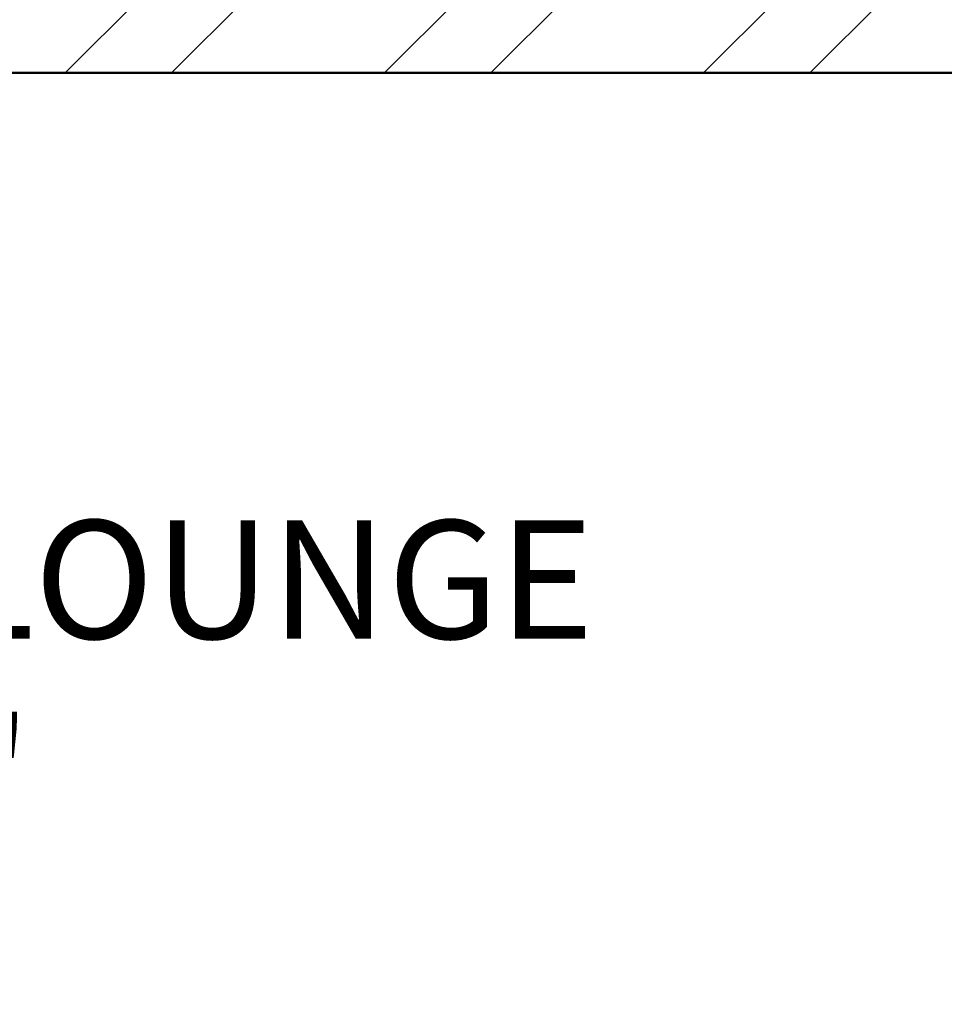
# Model space of a CAD drawing. Units: inches. Extents: x 963 to 2075, y 289 to 2657.
# Tile 91 of 98: x 1728 to 1767, y 2283 to 2325. Entities that reach past the tile are written whole.
import ezdxf

# ---------------------------------------------------------------- set-up
doc = ezdxf.new("R2010")
doc.units = ezdxf.units.IN
for name, color, linetype, lineweight in [('A-AREA-IDEN', 7, 'Continuous', 18), ('A-WALL', 7, 'Continuous', 50), ('A-WALL-PATT', 8, 'Continuous', 13)]:
    doc.layers.add(name, color=color, linetype=linetype, lineweight=lineweight)
doc.styles.get("Standard").update_dxf_attribs({"font": 'arial.ttf'})

msp = doc.modelspace()

# ---------------------------------------------------------------- hatches: boundary and pattern name
at = {"layer": 'A-WALL-PATT'}
h = msp.add_hatch(dxfattribs=at)
h.set_pattern_fill('ANSI32', color=256)
h.paths.add_polyline_path([(1296.922, 2558.318), (1203.922, 2558.318), (1203.922, 2493.818), (1191.533, 2493.818), (1191.533, 2489.318), (1211.063, 2489.318), (1211.063, 2492.02), (1211.063, 2493.818), (1208.422, 2493.818), (1208.422, 2553.818), (1292.422, 2553.818), (1292.422, 2538.863), (1296.922, 2538.863)])
h.paths.add_polyline_path([(1442.422, 2558.318), (1349.422, 2558.318), (1349.422, 2538.943), (1353.922, 2538.943), (1353.922, 2553.818), (1437.922, 2553.818), (1437.922, 2493.818), (1434.542, 2493.818), (1434.542, 2489.318), (1448.311, 2489.318), (1448.311, 2491.568), (1448.311, 2493.818), (1442.422, 2493.818)])
h.paths.add_polyline_path([(1415.554, 2491.568), (1415.554, 2493.818), (1340.941, 2493.818), (1340.941, 2489.318), (1371.922, 2489.318), (1371.922, 2378.318), (1367.596, 2378.318), (1367.596, 2373.818), (1371.922, 2373.818), (1371.922, 2355.185), (1376.422, 2355.185), (1376.422, 2489.318), (1415.554, 2489.318)])
h.paths.add_polyline_path([(1304.941, 2491.568), (1304.941, 2493.818), (1296.922, 2493.818), (1296.922, 2514.863), (1292.422, 2514.863), (1292.422, 2493.818), (1232.808, 2493.818), (1232.808, 2489.318), (1256.422, 2489.318), (1256.422, 2327.318), (1253.714, 2327.318), (1253.714, 2322.818), (1328.422, 2322.818), (1328.422, 2331.147), (1323.922, 2331.147), (1323.922, 2327.318), (1260.922, 2327.318), (1260.922, 2373.818), (1323.922, 2373.818), (1323.922, 2357.812), (1328.422, 2357.812), (1328.422, 2373.818), (1346.007, 2373.818), (1346.007, 2376.068), (1346.007, 2378.318), (1260.922, 2378.318), (1260.922, 2489.318), (1304.941, 2489.318)])
h.paths.add_polyline_path([(1226.654, 2327.318), (1124.422, 2327.318), (1124.422, 2347.447), (1119.922, 2347.447), (1119.922, 2322.818), (1163.422, 2322.818), (1163.422, 2305.435), (1165.672, 2305.435), (1167.922, 2305.435), (1167.922, 2322.818), (1226.654, 2322.818), (1226.654, 2325.068)])
h.paths.add_polyline_path([(1095.922, 2489.318), (1124.422, 2489.318), (1131.533, 2489.318), (1131.533, 2491.568), (1131.533, 2493.818), (1119.922, 2493.818), (1091.422, 2493.818), (1091.422, 2417.318), (1095.922, 2417.318), (1119.922, 2417.318), (1119.922, 2407.447), (1124.422, 2407.447), (1124.422, 2421.818), (1095.922, 2421.818)])
h.paths.add_polyline_path([(1512.922, 2558.318), (1508.422, 2558.318), (1508.422, 2493.818), (1503.401, 2493.818), (1503.401, 2489.318), (1508.422, 2489.318), (1508.422, 2327.318), (1376.422, 2327.318), (1376.422, 2330.273), (1371.922, 2330.273), (1371.922, 2298.744), (1376.422, 2298.744), (1376.422, 2322.818), (1508.422, 2322.818), (1508.422, 2165.318), (1504.255, 2165.318), (1504.255, 2160.818), (1508.422, 2160.818), (1508.422, 2108.318), (1512.922, 2108.318), (1512.922, 2160.818), (1516.182, 2160.818), (1516.182, 2163.068), (1516.182, 2165.318), (1512.922, 2165.318), (1512.922, 2322.818), (1644.922, 2322.818), (1644.922, 2298.744), (1649.422, 2298.744), (1649.422, 2322.818), (1649.422, 2330.944), (1647.172, 2330.944), (1644.922, 2330.944), (1644.922, 2327.318), (1512.922, 2327.318), (1512.922, 2489.318), (1516.759, 2489.318), (1516.759, 2491.568), (1516.759, 2493.818), (1512.922, 2493.818)])
h.paths.add_polyline_path([(1671.922, 2558.318), (1578.922, 2558.318), (1578.922, 2493.818), (1573.526, 2493.818), (1573.526, 2489.318), (1586.537, 2489.318), (1586.537, 2491.568), (1586.537, 2493.818), (1583.422, 2493.818), (1583.422, 2553.818), (1667.422, 2553.818), (1667.422, 2541.109), (1671.922, 2541.109)])
h.paths.add_polyline_path([(1681.257, 2493.818), (1671.922, 2493.818), (1671.922, 2517.109), (1667.422, 2517.109), (1667.422, 2493.818), (1610.218, 2493.818), (1610.218, 2489.318), (1644.922, 2489.318), (1644.922, 2357.865), (1649.422, 2357.865), (1649.422, 2373.818), (1652.203, 2373.818), (1652.203, 2375.827), (1652.203, 2378.318), (1649.422, 2378.318), (1649.422, 2489.318), (1681.257, 2489.318), (1681.257, 2491.568)])
h.paths.add_polyline_path([(1821.922, 2558.318), (1728.922, 2558.318), (1728.922, 2541), (1733.422, 2541), (1733.422, 2553.818), (1817.422, 2553.818), (1817.422, 2493.818), (1813.507, 2493.818), (1813.507, 2489.318), (1830.078, 2489.318), (1830.078, 2491.568), (1830.078, 2493.818), (1821.922, 2493.818)])
h.paths.add_polyline_path([(1794.244, 2493.818), (1717.257, 2493.818), (1717.257, 2489.318), (1760.422, 2489.318), (1760.422, 2378.318), (1674.401, 2378.318), (1674.401, 2373.818), (1692.922, 2373.818), (1692.922, 2356.954), (1697.422, 2356.954), (1697.422, 2373.818), (1760.422, 2373.818), (1760.422, 2327.318), (1697.422, 2327.318), (1697.422, 2333.341), (1692.922, 2333.341), (1692.922, 2322.818), (1768.037, 2322.818), (1768.037, 2325.068), (1768.037, 2327.318), (1764.922, 2327.318), (1764.922, 2489.318), (1794.244, 2489.318)])
h.paths.add_polyline_path([(1733.422, 2517), (1728.922, 2517), (1728.922, 2493.818), (1733.422, 2493.818)], flags=17)
h.paths.add_polyline_path([(1929.922, 2493.818), (1890.078, 2493.818), (1890.078, 2489.318), (1896.922, 2489.318), (1925.422, 2489.318), (1925.422, 2421.818), (1896.922, 2421.818), (1896.922, 2408.318), (1901.422, 2408.318), (1901.422, 2417.318), (1925.422, 2417.318), (1929.922, 2417.318)])
h.paths.add_polyline_path([(1901.422, 2348.318), (1896.922, 2348.318), (1896.922, 2327.318), (1800.423, 2327.318), (1800.423, 2322.818), (1853.422, 2322.818), (1853.422, 2309.453), (1857.922, 2309.453), (1857.922, 2322.818), (1901.422, 2322.818)])
h.paths.add_polyline_path([(1857.922, 2249.453), (1853.422, 2249.453), (1853.422, 2214.818), (1686.309, 2214.818), (1686.309, 2210.318), (1853.422, 2210.318), (1853.422, 2202.134), (1857.922, 2202.134), (1857.922, 2210.318)])
h.paths.add_polyline_path([(1857.922, 2142.134), (1853.422, 2142.134), (1853.422, 2115.422), (1841.422, 2115.422), (1841.422, 2088.531), (1841.422, 2046.949), (1845.922, 2046.949), (1845.922, 2110.922), (1905.922, 2110.922), (1905.922, 2092.517), (1910.422, 2092.517), (1910.422, 2115.422), (1857.922, 2115.422)])
h.paths.add_polyline_path([(1532.436, 1482.342), (1573.456, 1482.342), (1573.456, 1501), (1532.436, 1501)], flags=9)
h.paths.add_polyline_path([(1438.658, 1486.302), (1479.678, 1486.302), (1479.678, 1504.96), (1438.658, 1504.96)], flags=9)
h.paths.add_polyline_path([(1411.215, 1365.308), (1659.139, 1365.308), (1659.139, 1402.401), (1411.215, 1402.401)], flags=9)
h.paths.add_polyline_path([(1185.671, 2296.298), (1248.16, 2296.298), (1248.16, 2314.955), (1185.671, 2314.955)], flags=9)
h.paths.add_polyline_path([(1177.31, 2187.35), (1216.15, 2187.35), (1216.15, 2206.007), (1177.31, 2206.007)], flags=9)
h.paths.add_polyline_path([(1295.101, 1602.083), (1328.26, 1602.083), (1328.26, 1620.741), (1295.101, 1620.741)], flags=9)
h.paths.add_polyline_path([(1525.126, 2005.99), (1558.39, 2005.99), (1558.39, 2024.648), (1525.126, 2024.648)], flags=9)
h.paths.add_polyline_path([(1459.606, 1977.125), (1472.195, 1977.125), (1472.195, 1987.429), (1459.606, 1987.429)], flags=9)
h.paths.add_polyline_path([(1467.815, 2053.676), (1480.018, 2053.676), (1480.018, 2063.979), (1467.815, 2063.979)], flags=9)
h.paths.add_polyline_path([(1555.184, 2119.02), (1584.563, 2119.02), (1584.563, 2137.678), (1555.184, 2137.678)], flags=25)
h.paths.add_polyline_path([(1405.389, 2115.291), (1444.478, 2115.291), (1444.478, 2133.948), (1405.389, 2133.948)], flags=25)
h.paths.add_polyline_path([(1698.482, 2004.259), (1727.695, 2004.259), (1727.695, 2022.916), (1698.482, 2022.916)], flags=9)
h.paths.add_polyline_path([(1612.158, 1972.855), (1629.016, 1972.855), (1629.016, 1983.159), (1612.158, 1983.159)], flags=9)
h.paths.add_polyline_path([(1608.289, 2060.036), (1625.147, 2060.036), (1625.147, 2070.34), (1608.289, 2070.34)], flags=9)
h.paths.add_polyline_path([(1527.954, 1684.402), (1566.795, 1684.402), (1566.795, 1703.06), (1527.954, 1703.06)], flags=9)
h.paths.add_polyline_path([(1422.792, 1683.59), (1461.633, 1683.59), (1461.633, 1702.247), (1422.792, 1702.247)], flags=9)
h.paths.add_polyline_path([(1531.262, 1732.459), (1574.015, 1732.459), (1574.015, 1751.116), (1531.262, 1751.116)], flags=9)
h.paths.add_polyline_path([(1402.872, 1732.845), (1439.799, 1732.845), (1439.799, 1751.502), (1402.872, 1751.502)], flags=9)
h.paths.add_polyline_path([(1243.122, 1923.132), (1281.962, 1923.132), (1281.962, 1941.79), (1243.122, 1941.79)], flags=9)
h.paths.add_polyline_path([(1181.752, 1792.268), (1244.241, 1792.268), (1244.241, 1810.926), (1181.752, 1810.926)], flags=9)
h.paths.add_polyline_path([(1265.822, 1670.3), (1316.071, 1670.3), (1316.071, 1688.957), (1265.822, 1688.957)], flags=9)
h.paths.add_polyline_path([(1140.263, 1676.054), (1179.104, 1676.054), (1179.104, 1694.711), (1140.263, 1694.711)], flags=9)
h.paths.add_polyline_path([(1107.49, 1490.889), (1143.374, 1490.889), (1143.374, 1509.546), (1107.49, 1509.546)], flags=9)
h.paths.add_polyline_path([(1217.584, 1483.899), (1246.741, 1483.899), (1246.741, 1502.556), (1217.584, 1502.556)], flags=9)
h.paths.add_polyline_path([(1389.21, 1486.919), (1418.367, 1486.919), (1418.367, 1505.576), (1389.21, 1505.576)], flags=9)
h.paths.add_polyline_path([(1672.208, 1602.083), (1705.366, 1602.083), (1705.366, 1620.741), (1672.208, 1620.741)], flags=9)
h.paths.add_polyline_path([(1752.082, 1522.638), (1781.24, 1522.638), (1781.24, 1541.295), (1752.082, 1541.295)], flags=9)
h.paths.add_polyline_path([(1848.275, 1491.26), (1884.158, 1491.26), (1884.158, 1509.918), (1848.275, 1509.918)], flags=9)
h.paths.add_polyline_path([(1822.47, 1685.62), (1861.31, 1685.62), (1861.31, 1704.278), (1822.47, 1704.278)], flags=9)
h.paths.add_polyline_path([(1713.195, 1672.232), (1763.444, 1672.232), (1763.444, 1690.889), (1713.195, 1690.889)], flags=9)
h.paths.add_polyline_path([(1736.619, 1790.578), (1799.109, 1790.578), (1799.109, 1809.235), (1736.619, 1809.235)], flags=9)
h.paths.add_polyline_path([(1691.491, 1916.355), (1730.332, 1916.355), (1730.332, 1935.013), (1691.491, 1935.013)], flags=9)
h.paths.add_polyline_path([(1764.872, 1973.922), (1794.306, 1973.922), (1794.306, 1992.58), (1764.872, 1992.58)], flags=9)
h.paths.add_polyline_path([(1767.854, 2034.017), (1797.288, 2034.017), (1797.288, 2052.674), (1767.854, 2052.674)], flags=9)
h.paths.add_polyline_path([(1851.593, 2060.331), (1880.751, 2060.331), (1880.751, 2078.989), (1851.593, 2078.989)], flags=25)
h.paths.add_polyline_path([(1688.491, 2086.874), (1727.332, 2086.874), (1727.332, 2105.531), (1688.491, 2105.531)], flags=9)
h.paths.add_polyline_path([(1537.743, 2293.581), (1580.495, 2293.581), (1580.495, 2312.239), (1537.743, 2312.239)], flags=25)
h.paths.add_polyline_path([(1425.587, 2296.109), (1468.34, 2296.109), (1468.34, 2314.766), (1425.587, 2314.766)], flags=25)
h.paths.add_polyline_path([(1278.518, 2004.184), (1307.72, 2004.184), (1307.72, 2022.841), (1278.518, 2022.841)], flags=9)
h.paths.add_polyline_path([(1193.282, 1973.635), (1222.715, 1973.635), (1222.715, 1992.292), (1193.282, 1992.292)], flags=9)
h.paths.add_polyline_path([(1192.411, 2040.577), (1221.845, 2040.577), (1221.845, 2059.234), (1192.411, 2059.234)], flags=9)
h.paths.add_polyline_path([(1130.603, 1951.393), (1159.76, 1951.393), (1159.76, 1970.05), (1130.603, 1970.05)], flags=9)
h.paths.add_polyline_path([(1132.827, 2052.494), (1161.984, 2052.494), (1161.984, 2071.151), (1132.827, 2071.151)], flags=9)
h.paths.add_polyline_path([(1265.128, 2334.619), (1315.377, 2334.619), (1315.377, 2353.277), (1265.128, 2353.277)], flags=25)
h.paths.add_polyline_path([(1136.741, 2330.785), (1175.582, 2330.785), (1175.582, 2349.443), (1136.741, 2349.443)], flags=9)
h.paths.add_polyline_path([(1287.422, 2417.204), (1320.58, 2417.204), (1320.58, 2435.861), (1287.422, 2435.861)], flags=25)
h.paths.add_polyline_path([(1430.988, 2329.159), (1469.828, 2329.159), (1469.828, 2347.816), (1430.988, 2347.816)], flags=25)
h.paths.add_polyline_path([(1525.424, 2329.213), (1564.264, 2329.213), (1564.264, 2347.87), (1525.424, 2347.87)], flags=25)
h.paths.add_polyline_path([(1684.525, 2382.799), (1717.683, 2382.799), (1717.683, 2401.457), (1684.525, 2401.457)], flags=25)
h.paths.add_polyline_path([(1704.805, 2340.293), (1755.054, 2340.293), (1755.054, 2358.95), (1704.805, 2358.95)], flags=25)
h.paths.add_polyline_path([(1694.113, 2287.757), (1756.602, 2287.757), (1756.602, 2306.414), (1694.113, 2306.414)], flags=9)
h.paths.add_polyline_path([(1815.778, 2329.861), (1854.618, 2329.861), (1854.618, 2348.518), (1815.778, 2348.518)], flags=9)
h.paths.add_polyline_path([(1842.873, 2514.256), (1878.756, 2514.256), (1878.756, 2532.914), (1842.873, 2532.914)], flags=9)
h.paths.add_polyline_path([(1769.513, 2531.447), (1798.671, 2531.447), (1798.671, 2550.104), (1769.513, 2550.104)], flags=25)
h.paths.add_polyline_path([(1594.772, 2518.468), (1623.93, 2518.468), (1623.93, 2537.125), (1594.772, 2537.125)], flags=25)
h.paths.add_polyline_path([(1520.723, 2516.185), (1556.606, 2516.185), (1556.606, 2534.842), (1520.723, 2534.842)], flags=25)
h.paths.add_polyline_path([(1464.456, 2516.694), (1500.34, 2516.694), (1500.34, 2535.351), (1464.456, 2535.351)], flags=25)
h.paths.add_polyline_path([(1365.696, 2528.97), (1394.854, 2528.97), (1394.854, 2547.627), (1365.696, 2547.627)], flags=25)
h.paths.add_polyline_path([(1222.838, 2516.231), (1251.995, 2516.231), (1251.995, 2534.889), (1222.838, 2534.889)], flags=25)
h.paths.add_polyline_path([(1104.545, 2509.6), (1140.429, 2509.6), (1140.429, 2528.257), (1104.545, 2528.257)], flags=9)
h = msp.add_hatch(dxfattribs=at)
h.set_pattern_fill('ANSI32', color=256)
h.paths.add_polyline_path([(1335.968, 2212.568), (1335.968, 2214.818), (1167.922, 2214.818), (1167.922, 2245.435), (1163.422, 2245.435), (1163.422, 2210.318), (1163.422, 2194.812), (1167.922, 2194.812), (1167.922, 2210.318), (1335.968, 2210.318)])
h.paths.add_polyline_path([(1532.436, 1482.342), (1573.456, 1482.342), (1573.456, 1501), (1532.436, 1501)], flags=9)
h.paths.add_polyline_path([(1438.658, 1486.302), (1479.678, 1486.302), (1479.678, 1504.96), (1438.658, 1504.96)], flags=9)
h.paths.add_polyline_path([(1411.215, 1365.308), (1659.139, 1365.308), (1659.139, 1402.401), (1411.215, 1402.401)], flags=9)
h.paths.add_polyline_path([(1185.671, 2296.298), (1248.16, 2296.298), (1248.16, 2314.955), (1185.671, 2314.955)], flags=9)
h.paths.add_polyline_path([(1177.31, 2187.35), (1216.15, 2187.35), (1216.15, 2206.007), (1177.31, 2206.007)], flags=9)
h.paths.add_polyline_path([(1295.101, 1602.083), (1328.26, 1602.083), (1328.26, 1620.741), (1295.101, 1620.741)], flags=9)
h.paths.add_polyline_path([(1525.126, 2005.99), (1558.39, 2005.99), (1558.39, 2024.648), (1525.126, 2024.648)], flags=9)
h.paths.add_polyline_path([(1459.606, 1977.125), (1472.195, 1977.125), (1472.195, 1987.429), (1459.606, 1987.429)], flags=9)
h.paths.add_polyline_path([(1467.815, 2053.676), (1480.018, 2053.676), (1480.018, 2063.979), (1467.815, 2063.979)], flags=9)
h.paths.add_polyline_path([(1555.184, 2119.02), (1584.563, 2119.02), (1584.563, 2137.678), (1555.184, 2137.678)], flags=9)
h.paths.add_polyline_path([(1405.389, 2115.291), (1444.478, 2115.291), (1444.478, 2133.948), (1405.389, 2133.948)], flags=9)
h.paths.add_polyline_path([(1698.482, 2004.259), (1727.695, 2004.259), (1727.695, 2022.916), (1698.482, 2022.916)], flags=9)
h.paths.add_polyline_path([(1612.158, 1972.855), (1629.016, 1972.855), (1629.016, 1983.159), (1612.158, 1983.159)], flags=9)
h.paths.add_polyline_path([(1608.289, 2060.036), (1625.147, 2060.036), (1625.147, 2070.34), (1608.289, 2070.34)], flags=9)
h.paths.add_polyline_path([(1527.954, 1684.402), (1566.795, 1684.402), (1566.795, 1703.06), (1527.954, 1703.06)], flags=9)
h.paths.add_polyline_path([(1422.792, 1683.59), (1461.633, 1683.59), (1461.633, 1702.247), (1422.792, 1702.247)], flags=9)
h.paths.add_polyline_path([(1531.262, 1732.459), (1574.015, 1732.459), (1574.015, 1751.116), (1531.262, 1751.116)], flags=9)
h.paths.add_polyline_path([(1402.872, 1732.845), (1439.799, 1732.845), (1439.799, 1751.502), (1402.872, 1751.502)], flags=9)
h.paths.add_polyline_path([(1243.122, 1923.132), (1281.962, 1923.132), (1281.962, 1941.79), (1243.122, 1941.79)], flags=9)
h.paths.add_polyline_path([(1181.752, 1792.268), (1244.241, 1792.268), (1244.241, 1810.926), (1181.752, 1810.926)], flags=9)
h.paths.add_polyline_path([(1265.822, 1670.3), (1316.071, 1670.3), (1316.071, 1688.957), (1265.822, 1688.957)], flags=9)
h.paths.add_polyline_path([(1140.263, 1676.054), (1179.104, 1676.054), (1179.104, 1694.711), (1140.263, 1694.711)], flags=9)
h.paths.add_polyline_path([(1107.49, 1490.889), (1143.374, 1490.889), (1143.374, 1509.546), (1107.49, 1509.546)], flags=9)
h.paths.add_polyline_path([(1217.584, 1483.899), (1246.741, 1483.899), (1246.741, 1502.556), (1217.584, 1502.556)], flags=9)
h.paths.add_polyline_path([(1389.21, 1486.919), (1418.367, 1486.919), (1418.367, 1505.576), (1389.21, 1505.576)], flags=9)
h.paths.add_polyline_path([(1672.208, 1602.083), (1705.366, 1602.083), (1705.366, 1620.741), (1672.208, 1620.741)], flags=9)
h.paths.add_polyline_path([(1752.082, 1522.638), (1781.24, 1522.638), (1781.24, 1541.295), (1752.082, 1541.295)], flags=9)
h.paths.add_polyline_path([(1848.275, 1491.26), (1884.158, 1491.26), (1884.158, 1509.918), (1848.275, 1509.918)], flags=9)
h.paths.add_polyline_path([(1822.47, 1685.62), (1861.31, 1685.62), (1861.31, 1704.278), (1822.47, 1704.278)], flags=9)
h.paths.add_polyline_path([(1713.195, 1672.232), (1763.444, 1672.232), (1763.444, 1690.889), (1713.195, 1690.889)], flags=9)
h.paths.add_polyline_path([(1736.619, 1790.578), (1799.109, 1790.578), (1799.109, 1809.235), (1736.619, 1809.235)], flags=9)
h.paths.add_polyline_path([(1691.491, 1916.355), (1730.332, 1916.355), (1730.332, 1935.013), (1691.491, 1935.013)], flags=9)
h.paths.add_polyline_path([(1764.872, 1973.922), (1794.306, 1973.922), (1794.306, 1992.58), (1764.872, 1992.58)], flags=9)
h.paths.add_polyline_path([(1767.854, 2034.017), (1797.288, 2034.017), (1797.288, 2052.674), (1767.854, 2052.674)], flags=9)
h.paths.add_polyline_path([(1851.593, 2060.331), (1880.751, 2060.331), (1880.751, 2078.989), (1851.593, 2078.989)], flags=9)
h.paths.add_polyline_path([(1688.491, 2086.874), (1727.332, 2086.874), (1727.332, 2105.531), (1688.491, 2105.531)], flags=9)
h.paths.add_polyline_path([(1537.743, 2293.581), (1580.495, 2293.581), (1580.495, 2312.239), (1537.743, 2312.239)], flags=9)
h.paths.add_polyline_path([(1425.587, 2296.109), (1468.34, 2296.109), (1468.34, 2314.766), (1425.587, 2314.766)], flags=9)
h.paths.add_polyline_path([(1278.518, 2004.184), (1307.72, 2004.184), (1307.72, 2022.841), (1278.518, 2022.841)], flags=9)
h.paths.add_polyline_path([(1193.282, 1973.635), (1222.715, 1973.635), (1222.715, 1992.292), (1193.282, 1992.292)], flags=9)
h.paths.add_polyline_path([(1192.411, 2040.577), (1221.845, 2040.577), (1221.845, 2059.234), (1192.411, 2059.234)], flags=9)
h.paths.add_polyline_path([(1130.603, 1951.393), (1159.76, 1951.393), (1159.76, 1970.05), (1130.603, 1970.05)], flags=9)
h.paths.add_polyline_path([(1132.827, 2052.494), (1161.984, 2052.494), (1161.984, 2071.151), (1132.827, 2071.151)], flags=9)
h.paths.add_polyline_path([(1265.128, 2334.619), (1315.377, 2334.619), (1315.377, 2353.277), (1265.128, 2353.277)], flags=9)
h.paths.add_polyline_path([(1136.741, 2330.785), (1175.582, 2330.785), (1175.582, 2349.443), (1136.741, 2349.443)], flags=9)
h.paths.add_polyline_path([(1287.422, 2417.204), (1320.58, 2417.204), (1320.58, 2435.861), (1287.422, 2435.861)], flags=9)
h.paths.add_polyline_path([(1430.988, 2329.159), (1469.828, 2329.159), (1469.828, 2347.816), (1430.988, 2347.816)], flags=9)
h.paths.add_polyline_path([(1525.424, 2329.213), (1564.264, 2329.213), (1564.264, 2347.87), (1525.424, 2347.87)], flags=9)
h.paths.add_polyline_path([(1684.525, 2382.799), (1717.683, 2382.799), (1717.683, 2401.457), (1684.525, 2401.457)], flags=9)
h.paths.add_polyline_path([(1704.805, 2340.293), (1755.054, 2340.293), (1755.054, 2358.95), (1704.805, 2358.95)], flags=9)
h.paths.add_polyline_path([(1694.113, 2287.757), (1756.602, 2287.757), (1756.602, 2306.414), (1694.113, 2306.414)], flags=9)
h.paths.add_polyline_path([(1815.778, 2329.861), (1854.618, 2329.861), (1854.618, 2348.518), (1815.778, 2348.518)], flags=9)
h.paths.add_polyline_path([(1842.873, 2514.256), (1878.756, 2514.256), (1878.756, 2532.914), (1842.873, 2532.914)], flags=9)
h.paths.add_polyline_path([(1769.513, 2531.447), (1798.671, 2531.447), (1798.671, 2550.104), (1769.513, 2550.104)], flags=9)
h.paths.add_polyline_path([(1594.772, 2518.468), (1623.93, 2518.468), (1623.93, 2537.125), (1594.772, 2537.125)], flags=9)
h.paths.add_polyline_path([(1520.723, 2516.185), (1556.606, 2516.185), (1556.606, 2534.842), (1520.723, 2534.842)], flags=9)
h.paths.add_polyline_path([(1464.456, 2516.694), (1500.34, 2516.694), (1500.34, 2535.351), (1464.456, 2535.351)], flags=9)
h.paths.add_polyline_path([(1365.696, 2528.97), (1394.854, 2528.97), (1394.854, 2547.627), (1365.696, 2547.627)], flags=9)
h.paths.add_polyline_path([(1222.838, 2516.231), (1251.995, 2516.231), (1251.995, 2534.889), (1222.838, 2534.889)], flags=9)
h.paths.add_polyline_path([(1104.545, 2509.6), (1140.429, 2509.6), (1140.429, 2528.257), (1104.545, 2528.257)], flags=9)

# ---------------------------------------------------------------- linework, layer by layer
at = {"layer": 'A-WALL'}
msp.add_line((1692.922, 2322.818), (1768.037, 2322.818), dxfattribs=at)

# ---------------------------------------------------------------- texts
at = {"layer": 'A-AREA-IDEN', "insert": (1696.123, 2303.93), "char_height": 5, "attachment_point": 1}
msp.add_mtext_dynamic_manual_height_columns('DINING / LOUNGE\\P17\'0"x9\'0"', width=121.79467, gutter_width=12.5, heights=[0], dxfattribs=at)

doc.saveas('drawing.dxf')
